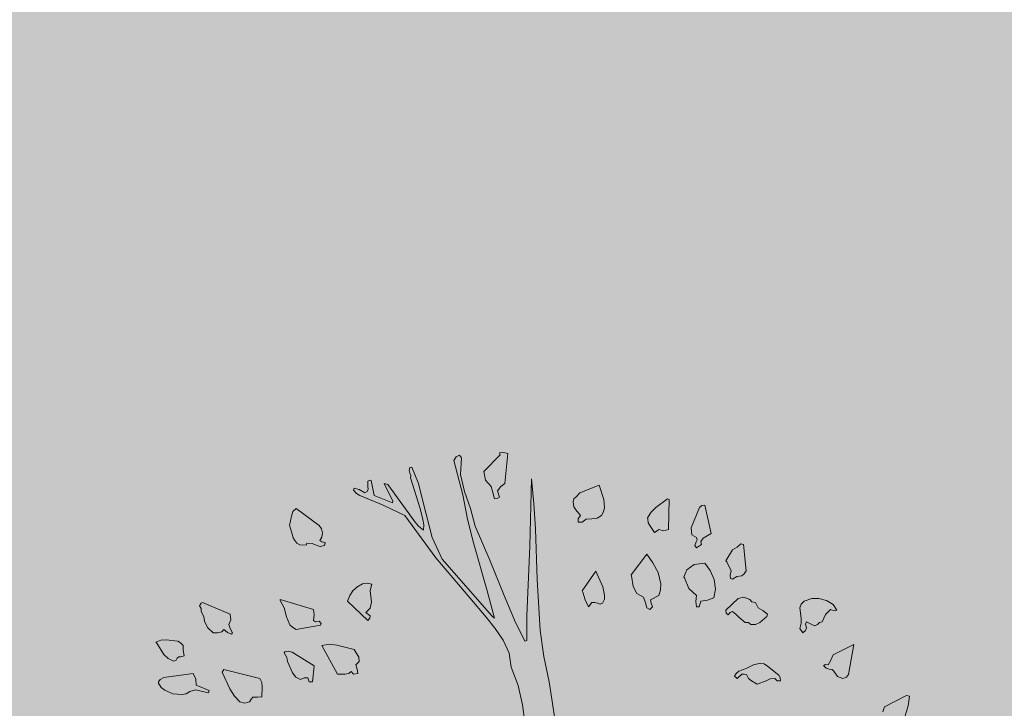
# Model space of a CAD drawing. Units: inches. Extents: x 84 to 1044, y -280 to 906.
# Tile 29 of 105: x 764 to 789, y -105 to -87. Entities that reach past the tile are written whole.
import ezdxf

# ---------------------------------------------------------------- set-up
doc = ezdxf.new("R2010")
doc.units = ezdxf.units.IN
doc.layers.add('L-PLNT', color=114, linetype='Continuous', lineweight=15)
doc.layers.add('L-PLNT-PATT', color=9, linetype='Continuous', lineweight=9, true_color=0xafd9aa)

# ---------------------------------------------------------------- blocks, each defined once
blk = doc.blocks.new('A$C37E508DF')
for p, q in [((0.7083, 1.5239), (0.7152, 1.5244)), ((0.7096, 1.5209), (0.7083, 1.5239)), ((0.7152, 1.5244), (0.7225, 1.5231)), ((0.7225, 1.5231), (0.7174, 1.4729)), ((0.6329, 1.5111), (0.6367, 1.5175)), ((0.6475, 1.4545), (0.6329, 1.5111)), ((0.6367, 1.5175), (0.6423, 1.5201)), ((0.6423, 1.5201), (0.6453, 1.5158)), ((0.6453, 1.5158), (0.644, 1.4879)), ((0.6826, 1.493), (0.7096, 1.5209)), ((0.5583, 1.4948), (0.5596, 1.4995)), ((0.5596, 1.4905), (0.5583, 1.4948)), ((0.5596, 1.4995), (0.563, 1.5003)), ((0.5613, 1.4862), (0.5596, 1.4905)), ((0.563, 1.5003), (0.5737, 1.4733)), ((0.6852, 1.4785), (0.6826, 1.493)), ((0.4897, 1.4772), (0.4935, 1.4789)), ((0.4897, 1.4678), (0.4897, 1.4772)), ((0.4935, 1.4789), (0.4952, 1.478)), ((0.4952, 1.478), (0.5004, 1.4532)), ((0.5313, 1.4437), (0.5167, 1.4729)), ((0.5167, 1.4729), (0.5231, 1.4716)), ((0.5608, 1.4823), (0.5613, 1.4862)), ((0.5767, 1.4317), (0.5608, 1.4823)), ((0.5737, 1.4733), (0.5814, 1.4437)), ((0.644, 1.4879), (0.6505, 1.46)), ((0.6946, 1.4682), (0.6852, 1.4785)), ((0.7174, 1.4729), (0.7109, 1.4682)), ((0.7589, 1.3691), (0.7615, 1.481)), ((0.7615, 1.481), (0.7658, 1.4395)), ((0.4657, 1.4622), (0.4669, 1.4652)), ((0.4708, 1.4566), (0.4657, 1.4622)), ((0.4669, 1.4652), (0.4755, 1.463)), ((0.4764, 1.4532), (0.4708, 1.4566)), ((0.4755, 1.463), (0.4845, 1.4575)), ((0.4845, 1.4575), (0.4884, 1.4596)), ((0.4884, 1.4596), (0.4905, 1.4635)), ((0.4905, 1.4635), (0.4897, 1.4678)), ((0.5231, 1.4716), (0.5686, 1.409)), ((0.6505, 1.46), (0.6603, 1.4317)), ((0.6976, 1.4579), (0.6946, 1.4682)), ((0.7002, 1.4476), (0.6976, 1.4579)), ((0.7109, 1.4682), (0.7053, 1.4609)), ((0.7053, 1.4609), (0.7083, 1.4502)), ((0.8357, 1.451), (0.8421, 1.4575)), ((0.8421, 1.4575), (0.8739, 1.4703)), ((0.8739, 1.4703), (0.882, 1.4463)), ((0.5154, 1.4373), (0.4764, 1.4532)), ((0.5004, 1.4532), (0.5308, 1.4412)), ((0.5308, 1.4412), (0.5313, 1.4437)), ((0.5814, 1.4437), (0.5969, 1.3833)), ((0.6552, 1.4137), (0.6475, 1.4545)), ((0.7049, 1.448), (0.7002, 1.4476)), ((0.7083, 1.4502), (0.7049, 1.448)), ((0.831, 1.4424), (0.8323, 1.4476)), ((0.8318, 1.4343), (0.831, 1.4424)), ((0.8323, 1.4476), (0.8357, 1.451)), ((0.882, 1.4463), (0.8829, 1.433)), ((0.9686, 1.4334), (0.9875, 1.4476)), ((0.9875, 1.4476), (0.9905, 1.4467)), ((0.9905, 1.4467), (0.9896, 1.3966)), ((0.3628, 1.4189), (0.3649, 1.4266)), ((0.3649, 1.4266), (0.3709, 1.4317)), ((0.3709, 1.4317), (0.4086, 1.403)), ((0.551, 1.4197), (0.5154, 1.4373)), ((0.5814, 1.4133), (0.5767, 1.4317)), ((0.6603, 1.4317), (0.668, 1.4021)), ((0.7658, 1.4395), (0.7684, 1.3979)), ((0.8353, 1.4292), (0.8318, 1.4343)), ((0.8434, 1.4197), (0.8353, 1.4292)), ((0.8816, 1.4262), (0.8781, 1.4197)), ((0.8829, 1.433), (0.8816, 1.4262)), ((0.9545, 1.4159), (0.9605, 1.4257)), ((0.9605, 1.4257), (0.9686, 1.4334)), ((1.0269, 1.3996), (1.0411, 1.433)), ((1.0411, 1.433), (1.045, 1.4365)), ((1.045, 1.4365), (1.0497, 1.4369)), ((1.0497, 1.4369), (1.0604, 1.3901)), ((0.3598, 1.403), (0.3628, 1.4189)), ((0.6029, 1.3494), (0.551, 1.4197)), ((0.5686, 1.409), (0.5741, 1.4021)), ((0.5827, 1.4043), (0.5814, 1.4133)), ((0.6655, 1.3743), (0.6552, 1.4137)), ((0.8391, 1.4141), (0.8434, 1.4197)), ((0.8395, 1.4086), (0.8391, 1.4141)), ((0.846, 1.4086), (0.8395, 1.4086)), ((0.8528, 1.4137), (0.846, 1.4086)), ((0.8619, 1.4146), (0.8528, 1.4137)), ((0.8709, 1.4154), (0.8619, 1.4146)), ((0.8781, 1.4197), (0.8709, 1.4154)), ((0.9549, 1.4146), (0.9545, 1.4159)), ((0.9558, 1.4077), (0.9549, 1.4146)), ((0.9592, 1.4017), (0.9558, 1.4077)), ((0.3602, 1.4021), (0.3598, 1.403)), ((0.364, 1.3888), (0.3602, 1.4021)), ((0.4086, 1.403), (0.4125, 1.3979)), ((0.4125, 1.3979), (0.4142, 1.391)), ((0.4142, 1.391), (0.4134, 1.3837)), ((0.5741, 1.4021), (0.5823, 1.3953)), ((0.5823, 1.3953), (0.5827, 1.4043)), ((0.668, 1.4021), (0.6925, 1.3455)), ((0.7684, 1.3979), (0.771, 1.3134)), ((0.966, 1.3914), (0.9592, 1.4017)), ((0.9703, 1.3944), (0.966, 1.3914)), ((0.9733, 1.3966), (0.9703, 1.3944)), ((0.9819, 1.3944), (0.9733, 1.3966)), ((0.9896, 1.3966), (0.9819, 1.3944)), ((1.0282, 1.3876), (1.0269, 1.3996)), ((0.3657, 1.3828), (0.364, 1.3888)), ((0.3683, 1.3781), (0.3657, 1.3828)), ((0.3718, 1.3738), (0.3683, 1.3781)), ((0.4134, 1.3837), (0.4099, 1.3781)), ((0.4099, 1.3781), (0.4134, 1.376)), ((0.4134, 1.376), (0.4189, 1.3751)), ((0.4189, 1.3751), (0.4176, 1.37)), ((0.5969, 1.3833), (0.6132, 1.3472)), ((1.0359, 1.3833), (1.0282, 1.3876)), ((1.0334, 1.37), (1.0351, 1.376)), ((1.0351, 1.376), (1.0368, 1.3794)), ((1.0368, 1.3794), (1.0359, 1.3833)), ((1.0471, 1.3824), (1.0432, 1.3764)), ((1.0432, 1.3764), (1.0441, 1.3717)), ((1.0604, 1.3901), (1.0471, 1.3824)), ((0.3765, 1.3713), (0.3718, 1.3738)), ((0.3872, 1.3708), (0.3765, 1.3713)), ((0.3885, 1.3738), (0.3872, 1.3708)), ((0.3971, 1.3734), (0.3885, 1.3738)), ((0.4039, 1.3704), (0.3971, 1.3734)), ((0.4108, 1.3683), (0.4039, 1.3704)), ((0.4176, 1.37), (0.4108, 1.3683)), ((0.6882, 1.2949), (0.6655, 1.3743)), ((0.7538, 1.2529), (0.7589, 1.3691)), ((1.0359, 1.3661), (1.0334, 1.37)), ((1.0441, 1.3717), (1.0359, 1.3661)), ((1.0848, 1.3443), (1.0955, 1.3631)), ((1.0955, 1.3631), (1.1033, 1.367)), ((1.1033, 1.367), (1.1097, 1.373)), ((1.1097, 1.373), (1.114, 1.3717)), ((1.114, 1.3717), (1.1183, 1.328)), ((0.6595, 1.2829), (0.6029, 1.3494)), ((0.6132, 1.3472), (0.6959, 1.2529)), ((0.6925, 1.3455), (0.7161, 1.2868)), ((0.9274, 1.3215), (0.9532, 1.3554)), ((0.9532, 1.3554), (0.9635, 1.3413)), ((1.0861, 1.343), (1.0848, 1.3443)), ((1.0938, 1.328), (1.0861, 1.343)), ((0.846, 1.2949), (0.8687, 1.3271)), ((0.8687, 1.3271), (0.8803, 1.3014)), ((0.9635, 1.3413), (0.9721, 1.325)), ((1.0171, 1.3232), (1.0197, 1.3297)), ((1.0197, 1.3297), (1.0321, 1.3387)), ((1.0321, 1.3387), (1.0497, 1.3404)), ((1.0497, 1.3404), (1.0587, 1.3284)), ((1.0587, 1.3284), (1.0651, 1.3134)), ((1.0917, 1.3207), (1.0938, 1.328)), ((1.1183, 1.328), (1.1153, 1.3228)), ((0.771, 1.3134), (0.7761, 1.2285)), ((0.9279, 1.3194), (0.9274, 1.3215)), ((0.9305, 1.3018), (0.9279, 1.3194)), ((0.9721, 1.325), (0.9768, 1.3061)), ((1.0149, 1.3172), (1.0171, 1.3232)), ((1.0162, 1.3164), (1.0149, 1.3172)), ((1.0231, 1.2988), (1.0162, 1.3164)), ((1.0651, 1.3134), (1.0677, 1.2975)), ((1.0925, 1.3151), (1.0917, 1.3207)), ((1.0955, 1.3138), (1.0925, 1.3151)), ((1.1028, 1.3185), (1.0955, 1.3138)), ((1.111, 1.3194), (1.1028, 1.3185)), ((1.1153, 1.3228), (1.111, 1.3194)), ((0.4597, 1.2868), (0.4648, 1.2945)), ((0.4648, 1.2945), (0.4717, 1.3009)), ((0.4717, 1.3009), (0.4807, 1.3065)), ((0.4807, 1.3065), (0.4884, 1.3074)), ((0.4884, 1.3074), (0.4965, 1.3057)), ((0.4965, 1.3057), (0.4935, 1.2954)), ((0.4935, 1.2954), (0.4948, 1.2855)), ((0.7002, 1.2495), (0.6882, 1.2949)), ((0.8473, 1.2924), (0.846, 1.2949)), ((0.8803, 1.3014), (0.8833, 1.2872)), ((0.9365, 1.2902), (0.9305, 1.3018)), ((0.9763, 1.2962), (0.9733, 1.2868)), ((0.9768, 1.3061), (0.9763, 1.2962)), ((1.0359, 1.2868), (1.0231, 1.2988)), ((1.0677, 1.2975), (1.0647, 1.2829)), ((0.3439, 1.2804), (0.3992, 1.2636)), ((0.3439, 1.2787), (0.3439, 1.2804)), ((0.3507, 1.2662), (0.3439, 1.2787)), ((0.4562, 1.2774), (0.4597, 1.2868)), ((0.4897, 1.2452), (0.4562, 1.2774)), ((0.4948, 1.2855), (0.4961, 1.2756)), ((0.6865, 1.2508), (0.6595, 1.2829)), ((0.7161, 1.2868), (0.7349, 1.2422)), ((0.8507, 1.2795), (0.8473, 1.2924)), ((0.8567, 1.2679), (0.8507, 1.2795)), ((0.8829, 1.2808), (0.8799, 1.2744)), ((0.8833, 1.2872), (0.8829, 1.2808)), ((0.9476, 1.2842), (0.9365, 1.2902)), ((0.951, 1.2748), (0.9476, 1.2842)), ((0.9733, 1.2868), (0.9596, 1.2799)), ((0.9596, 1.2799), (0.9605, 1.2744)), ((1.0347, 1.2769), (1.0359, 1.2868)), ((1.0359, 1.2679), (1.0347, 1.2769)), ((1.0432, 1.2774), (1.0402, 1.2679)), ((1.0544, 1.2791), (1.0432, 1.2774)), ((1.0647, 1.2829), (1.0544, 1.2791)), ((1.0848, 1.2628), (1.1054, 1.2817)), ((1.1054, 1.2817), (1.1148, 1.2842)), ((1.1148, 1.2842), (1.1247, 1.2804)), ((1.1247, 1.2804), (1.1281, 1.2765)), ((1.1281, 1.2765), (1.1341, 1.2752)), ((1.21, 1.2726), (1.2147, 1.2774)), ((1.2147, 1.2774), (1.2276, 1.2817)), ((1.2276, 1.2817), (1.2392, 1.2817)), ((1.2392, 1.2817), (1.2521, 1.2787)), ((1.2521, 1.2787), (1.2632, 1.2722)), ((0.2101, 1.2696), (0.2127, 1.2744)), ((0.2127, 1.2654), (0.2101, 1.2696)), ((0.2127, 1.2744), (0.2152, 1.2752)), ((0.2127, 1.2602), (0.2127, 1.2654)), ((0.2174, 1.2521), (0.2127, 1.2602)), ((0.2152, 1.2752), (0.2611, 1.2559)), ((0.3546, 1.2516), (0.3507, 1.2662)), ((0.3992, 1.2636), (0.4005, 1.2546)), ((0.4935, 1.2658), (0.4867, 1.2589)), ((0.4961, 1.2756), (0.4935, 1.2658)), ((0.8619, 1.2752), (0.8567, 1.2679)), ((0.867, 1.2752), (0.8619, 1.2752)), ((0.8713, 1.2739), (0.867, 1.2752)), ((0.8756, 1.2726), (0.8713, 1.2739)), ((0.8799, 1.2744), (0.8756, 1.2726)), ((0.9532, 1.2666), (0.951, 1.2748)), ((0.9583, 1.2636), (0.9532, 1.2666)), ((0.9626, 1.2679), (0.9583, 1.2636)), ((0.9605, 1.2744), (0.9626, 1.2679)), ((1.0402, 1.2679), (1.0359, 1.2679)), ((1.0852, 1.2576), (1.0848, 1.2628)), ((1.0955, 1.2602), (1.0921, 1.2585)), ((1.1015, 1.2559), (1.0955, 1.2602)), ((1.1341, 1.2752), (1.1384, 1.2666)), ((1.1384, 1.2666), (1.1461, 1.2619)), ((1.1461, 1.2619), (1.1539, 1.2559)), ((1.2075, 1.2666), (1.21, 1.2726)), ((1.2096, 1.2491), (1.2075, 1.2666)), ((1.2585, 1.2636), (1.2503, 1.2551)), ((1.2645, 1.2615), (1.2585, 1.2636)), ((1.2632, 1.2722), (1.2692, 1.2628)), ((1.2692, 1.2628), (1.2645, 1.2615)), ((0.2182, 1.2443), (0.2174, 1.2521)), ((0.2234, 1.2336), (0.2182, 1.2443)), ((0.262, 1.2465), (0.2586, 1.2388)), ((0.2611, 1.2559), (0.262, 1.2465)), ((0.3602, 1.2383), (0.3546, 1.2516)), ((0.4005, 1.2546), (0.3992, 1.2452)), ((0.3992, 1.2452), (0.4026, 1.2431)), ((0.4026, 1.2431), (0.4086, 1.2443)), ((0.4086, 1.2443), (0.4121, 1.2401)), ((0.4867, 1.2589), (0.4935, 1.2529)), ((0.4931, 1.2491), (0.4897, 1.2452)), ((0.4935, 1.2529), (0.4931, 1.2491)), ((0.7015, 1.2323), (0.6865, 1.2508)), ((0.6959, 1.2529), (0.7002, 1.2495)), ((0.7538, 1.2122), (0.7538, 1.2529)), ((1.0883, 1.2546), (1.0852, 1.2576)), ((1.0921, 1.2585), (1.0883, 1.2546)), ((1.1063, 1.2508), (1.1015, 1.2559)), ((1.117, 1.2422), (1.1063, 1.2508)), ((1.1526, 1.2521), (1.141, 1.2422)), ((1.1539, 1.2559), (1.1526, 1.2521)), ((1.21, 1.2409), (1.2096, 1.2491)), ((1.2503, 1.2551), (1.2448, 1.2431)), ((0.2328, 1.2251), (0.2234, 1.2336)), ((0.2504, 1.2306), (0.2474, 1.2268)), ((0.2568, 1.2255), (0.2504, 1.2306)), ((0.2586, 1.2388), (0.2611, 1.2319)), ((0.2611, 1.2319), (0.265, 1.2251)), ((0.3649, 1.2336), (0.3602, 1.2383)), ((0.3709, 1.2306), (0.3649, 1.2336)), ((0.4112, 1.2375), (0.3709, 1.2306)), ((0.4121, 1.2401), (0.4112, 1.2375)), ((0.7148, 1.2126), (0.7015, 1.2323)), ((0.7349, 1.2422), (0.7482, 1.216)), ((0.7761, 1.2285), (0.7821, 1.1856)), ((1.1221, 1.2418), (1.117, 1.2422)), ((1.126, 1.2388), (1.1221, 1.2418)), ((1.1337, 1.2388), (1.126, 1.2388)), ((1.141, 1.2422), (1.1337, 1.2388)), ((1.2079, 1.2323), (1.21, 1.2409)), ((1.2126, 1.2251), (1.2079, 1.2323)), ((1.2169, 1.2285), (1.2126, 1.2251)), ((1.2186, 1.2332), (1.2169, 1.2285)), ((1.2186, 1.2431), (1.2173, 1.2392)), ((1.2173, 1.2392), (1.2186, 1.2332)), ((1.2285, 1.2383), (1.2186, 1.2431)), ((1.2328, 1.2366), (1.2285, 1.2383)), ((1.2371, 1.2388), (1.2328, 1.2366)), ((1.2405, 1.2418), (1.2371, 1.2388)), ((1.2448, 1.2431), (1.2405, 1.2418)), ((0.1376, 1.2092), (0.1458, 1.2126)), ((0.1458, 1.2126), (0.1548, 1.2135)), ((0.1548, 1.2135), (0.1741, 1.2109)), ((0.1741, 1.2109), (0.1784, 1.2083)), ((0.2401, 1.2251), (0.2328, 1.2251)), ((0.2474, 1.2268), (0.2401, 1.2251)), ((0.2633, 1.2229), (0.2568, 1.2255)), ((0.265, 1.2251), (0.2633, 1.2229)), ((0.7246, 1.1908), (0.7148, 1.2126)), ((0.7482, 1.216), (0.7508, 1.2109)), ((0.7508, 1.2109), (0.7538, 1.2122)), ((0.1389, 1.2079), (0.1376, 1.2092)), ((0.1505, 1.189), (0.1389, 1.2079)), ((0.1784, 1.2083), (0.1831, 1.204)), ((0.1831, 1.204), (0.1831, 1.1959)), ((0.1831, 1.1959), (0.1848, 1.1865)), ((0.4134, 1.204), (0.4258, 1.2058)), ((0.4391, 1.156), (0.4134, 1.204)), ((0.4258, 1.2058), (0.4382, 1.2045)), ((0.4382, 1.2045), (0.4669, 1.1972)), ((0.4669, 1.1972), (0.4747, 1.1843)), ((1.2628, 1.1882), (1.2975, 1.2053)), ((1.2975, 1.2053), (1.2885, 1.1556)), ((0.1582, 1.1822), (0.1505, 1.189)), ((0.1668, 1.1775), (0.1582, 1.1822)), ((0.1711, 1.1792), (0.1668, 1.1775)), ((0.1728, 1.1826), (0.1711, 1.1792)), ((0.1758, 1.1847), (0.1728, 1.1826)), ((0.1788, 1.1852), (0.1758, 1.1847)), ((0.1848, 1.1865), (0.1788, 1.1852)), ((0.3507, 1.1916), (0.352, 1.1933)), ((0.355, 1.1839), (0.3507, 1.1916)), ((0.352, 1.1933), (0.3576, 1.1942)), ((0.3563, 1.177), (0.355, 1.1839)), ((0.3576, 1.1942), (0.364, 1.1929)), ((0.364, 1.1929), (0.4005, 1.1702)), ((0.4747, 1.1843), (0.4751, 1.177)), ((0.7281, 1.168), (0.7246, 1.1908)), ((0.7821, 1.1856), (0.7911, 1.1436)), ((1.2546, 1.1719), (1.2589, 1.1792)), ((1.2589, 1.1792), (1.2628, 1.1882)), ((0.2478, 1.1594), (0.2504, 1.1637)), ((0.2504, 1.1637), (0.3104, 1.1487)), ((0.3645, 1.1586), (0.3563, 1.177)), ((0.4005, 1.1702), (0.3979, 1.1436)), ((0.4751, 1.177), (0.47, 1.1714)), ((0.47, 1.1714), (0.4721, 1.1646)), ((0.4721, 1.1646), (0.473, 1.1573)), ((0.7396, 1.1371), (0.7281, 1.168)), ((1.1063, 1.1612), (1.1187, 1.1655)), ((1.1187, 1.1655), (1.1307, 1.1714)), ((1.1307, 1.1714), (1.1423, 1.1744)), ((1.1423, 1.1744), (1.1483, 1.1732)), ((1.1483, 1.1732), (1.1539, 1.1693)), ((1.1539, 1.1693), (1.1727, 1.1543)), ((1.2469, 1.1702), (1.2495, 1.1723)), ((1.2478, 1.1693), (1.2469, 1.1702)), ((1.2516, 1.1659), (1.2478, 1.1693)), ((1.2495, 1.1723), (1.2546, 1.1719)), ((1.2563, 1.1646), (1.2516, 1.1659)), ((1.2611, 1.1637), (1.2563, 1.1646)), ((1.2641, 1.1612), (1.2611, 1.1637)), ((0.1419, 1.1436), (0.1449, 1.1474)), ((0.1449, 1.1474), (0.1509, 1.1504)), ((0.1509, 1.1504), (0.1994, 1.1573)), ((0.1994, 1.1573), (0.2041, 1.1479)), ((0.2041, 1.1479), (0.2045, 1.138)), ((0.2607, 1.1316), (0.2478, 1.1594)), ((0.3104, 1.1487), (0.3134, 1.1423)), ((0.37, 1.1509), (0.3645, 1.1586)), ((0.3778, 1.1474), (0.37, 1.1509)), ((0.3842, 1.15), (0.3778, 1.1474)), ((0.3898, 1.15), (0.3842, 1.15)), ((0.3923, 1.1436), (0.3898, 1.15)), ((0.4519, 1.1564), (0.4391, 1.156)), ((0.458, 1.1573), (0.4519, 1.1564)), ((0.4622, 1.1607), (0.458, 1.1573)), ((0.4657, 1.156), (0.4622, 1.1607)), ((0.473, 1.1573), (0.4657, 1.156)), ((1.099, 1.153), (1.102, 1.1573)), ((1.1033, 1.1487), (1.099, 1.153)), ((1.102, 1.1573), (1.1063, 1.1612)), ((1.111, 1.156), (1.1033, 1.1487)), ((1.1153, 1.1564), (1.111, 1.156)), ((1.1191, 1.1556), (1.1153, 1.1564)), ((1.1226, 1.1492), (1.1191, 1.1556)), ((1.1273, 1.1453), (1.1226, 1.1492)), ((1.1586, 1.1483), (1.1517, 1.1453)), ((1.1663, 1.1487), (1.1586, 1.1483)), ((1.1697, 1.1449), (1.1663, 1.1487)), ((1.1727, 1.1543), (1.1749, 1.1504)), ((1.1749, 1.1504), (1.1757, 1.1449)), ((1.2701, 1.1522), (1.2641, 1.1612)), ((1.2791, 1.1487), (1.2701, 1.1522)), ((1.2851, 1.1509), (1.2791, 1.1487)), ((1.2885, 1.1556), (1.2851, 1.1509)), ((0.1419, 1.141), (0.1419, 1.1436)), ((0.1462, 1.1342), (0.1419, 1.141)), ((0.1522, 1.1294), (0.1462, 1.1342)), ((0.1655, 1.1234), (0.1522, 1.1294)), ((0.2032, 1.1303), (0.1938, 1.1273)), ((0.2247, 1.1251), (0.2032, 1.1303)), ((0.2045, 1.138), (0.226, 1.129)), ((0.226, 1.129), (0.2247, 1.1251)), ((0.268, 1.1196), (0.2607, 1.1316)), ((0.3134, 1.1423), (0.3139, 1.1346)), ((0.3139, 1.1346), (0.3134, 1.1183)), ((0.3979, 1.1436), (0.3923, 1.1436)), ((0.7469, 1.1054), (0.7396, 1.1371)), ((0.7911, 1.1436), (0.8027, 1.0677)), ((1.1367, 1.1393), (1.1273, 1.1453)), ((1.1517, 1.1453), (1.1367, 1.1393)), ((1.1757, 1.1449), (1.1697, 1.1449)), ((0.181, 1.1226), (0.1655, 1.1234)), ((0.1878, 1.1234), (0.181, 1.1226)), ((0.1938, 1.1273), (0.1878, 1.1234)), ((0.277, 1.1101), (0.268, 1.1196)), ((0.2959, 1.1144), (0.2933, 1.1101)), ((0.2984, 1.1179), (0.2959, 1.1144)), ((0.3066, 1.1179), (0.2984, 1.1179)), ((0.3134, 1.1183), (0.3066, 1.1179)), ((1.3485, 1.102), (1.385, 1.1209)), ((1.385, 1.1209), (1.3897, 1.1196)), ((1.3897, 1.1196), (1.3875, 1.1037)), ((0.2856, 1.108), (0.277, 1.1101)), ((0.2933, 1.1101), (0.2856, 1.108)), ((0.7512, 1.0728), (0.7469, 1.1054)), ((1.3455, 1.0934), (1.3485, 1.102)), ((1.3875, 1.1037), (1.3828, 1.087))]:
    blk.add_line(p, q)

msp = doc.modelspace()

# ---------------------------------------------------------------- hatches: boundary and pattern name
at = {"layer": 'L-PLNT-PATT', "transparency": 33554597}
h = msp.add_hatch(color=256, dxfattribs=at)
h.dxf.hatch_style = 1
h.paths.add_polyline_path([(791.074, 31.12), (791.074, 91.12), (743.074, 91.12), (674.074, 91.12), (674.074, 31.12), (650.074, 31.12), (650.074, -112.88), (983.074, -112.88), (983.074, -64.88), (791.074, -64.88)])

# ---------------------------------------------------------------- block references
at = {"layer": 'L-PLNT', "xscale": 15.19586232982809, "yscale": 15.19586232982809, "zscale": 15.19586232982809}
msp.add_blockref('A$C37E508DF', (765.534, -121.265), dxfattribs=at)

doc.saveas('drawing.dxf')
